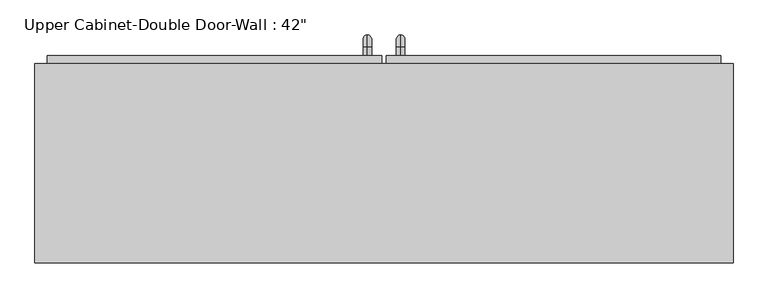
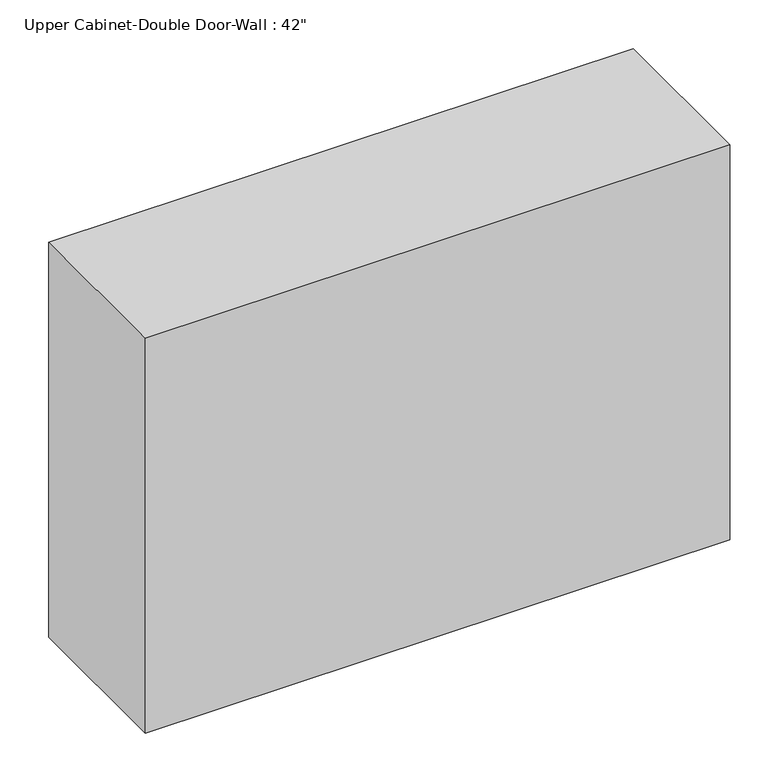
"""IFC4 building model written with IfcOpenShell, lengths in millimetres: furniture geometry."""

from ifc_helpers import new_model, si_unit, point, frame, origin, place, context, project, spatial, polyline, circle_curve, ellipse_curve, trimmed, outline, extrude, faceted_brep, source, transform, mapped, element, save
from ifc_brep_helpers import plane_surface, cylinder_surface, revolved_surface, advanced_brep


def furniture_f73e1c42(model_context):
    return source(origin(), model_context, "Body", "SolidModel", [
        extrude(outline(polyline([(32.9461628, 374.65), (544.1211628, 374.65), (544.1211628, 342.9), (32.9461628, 342.9), (32.9461628, 374.65)])), frame((0.0, 0.0, 1390.65), z_axis=(0.0, 0.0, 1.0), x_axis=(1.0, 0.0, 0.0)), (0.0, 0.0, 1.0), 723.9),
        extrude(outline(polyline([(-484.5788372, 374.65), (26.5961628, 374.65), (26.5961628, 342.9), (-484.5788372, 342.9), (-484.5788372, 374.65)])), frame((0.0, 0.0, 1390.65), z_axis=(0.0, 0.0, 1.0), x_axis=(1.0, 0.0, 0.0)), (0.0, 0.0, 1.0), 723.9),
        advanced_brep(
        [(4.3711628, 374.65, 1517.65), (4.3711628, 374.65, 1530.35), (4.3711628, 387.35, 1517.65), (4.3711628, 387.35, 1530.35), (4.3711628, 406.4, 1511.3), (4.3711628, 393.7, 1511.3), (4.3711628, 393.7, 1435.1), (4.3711628, 406.4, 1435.1), (4.3711628, 387.35, 1416.05), (4.3711628, 387.35, 1428.75), (4.3711628, 374.65, 1428.75), (4.3711628, 374.65, 1416.05)],
        [
            (0, 1, circle_curve(frame((4.3711628, 374.65, 1524.0), z_axis=(0.0, -1.0, 0.0), x_axis=(0.0, 0.0, 1.0)), 6.35)),
            (1, 0, circle_curve(frame((4.3711628, 374.65, 1524.0), z_axis=(0.0, -1.0, 0.0), x_axis=(0.0, 0.0, 1.0)), 6.35)),
            (0, 2),
            (2, 3, circle_curve(frame((4.3711628, 387.35, 1524.0), z_axis=(0.0, -1.0, 0.0), x_axis=(0.0, 0.0, 1.0)), 6.35)),
            (3, 1),
            (3, 2, circle_curve(frame((4.3711628, 387.35, 1524.0), z_axis=(0.0, -1.0, 0.0), x_axis=(0.0, 0.0, 1.0)), 6.35)),
            (4, 3, circle_curve(frame((4.3711628, 387.35, 1511.3), z_axis=(1.0, 0.0, 0.0), x_axis=(0.0, 0.0, 1.0)), 19.05)),
            (2, 5, circle_curve(frame((4.3711628, 387.35, 1511.3), z_axis=(-1.0, 0.0, 0.0), x_axis=(0.0, 0.0, 1.0)), 6.35)),
            (5, 4, circle_curve(frame((4.3711628, 400.05, 1511.3), z_axis=(0.0, 0.0, 1.0), x_axis=(0.0, 1.0, 0.0)), 6.35)),
            (4, 5, circle_curve(frame((4.3711628, 400.05, 1511.3), z_axis=(0.0, 0.0, 1.0), x_axis=(0.0, 1.0, 0.0)), 6.35)),
            (5, 6),
            (6, 7, circle_curve(frame((4.3711628, 400.05, 1435.1), z_axis=(0.0, 0.0, 1.0), x_axis=(0.0, 1.0, 0.0)), 6.35)),
            (7, 4),
            (7, 6, circle_curve(frame((4.3711628, 400.05, 1435.1), z_axis=(0.0, 0.0, 1.0), x_axis=(0.0, 1.0, 0.0)), 6.35)),
            (8, 7, circle_curve(frame((4.3711628, 387.35, 1435.1), z_axis=(1.0, 0.0, 0.0), x_axis=(0.0, 1.0, 0.0)), 19.05)),
            (6, 9, circle_curve(frame((4.3711628, 387.35, 1435.1), z_axis=(-1.0, 0.0, 0.0), x_axis=(0.0, 1.0, 0.0)), 6.35)),
            (9, 8, circle_curve(frame((4.3711628, 387.35, 1422.4), z_axis=(0.0, 1.0, 0.0), x_axis=(0.0, 0.0, -1.0)), 6.35)),
            (8, 9, circle_curve(frame((4.3711628, 387.35, 1422.4), z_axis=(0.0, 1.0, 0.0), x_axis=(0.0, 0.0, -1.0)), 6.35)),
            (10, 11, circle_curve(frame((4.3711628, 374.65, 1422.4), z_axis=(0.0, -1.0, 0.0), x_axis=(0.0, 0.0, -1.0)), 6.35)),
            (11, 10, circle_curve(frame((4.3711628, 374.65, 1422.4), z_axis=(0.0, -1.0, 0.0), x_axis=(0.0, 0.0, -1.0)), 6.35)),
            (9, 10),
            (11, 8),
        ],
        [
            plane_surface(frame((-1.9788372, 374.65, 1524.0), z_axis=(0.0, -1.0, 0.0), x_axis=(0.0, 0.0, 1.0))),
            cylinder_surface(frame((4.3711628, 374.65, 1524.0), z_axis=(0.0, -1.0, 0.0), x_axis=(0.0, 0.0, 1.0)), 6.35),
            revolved_surface(trimmed(ellipse_curve(frame((4.3711628, 387.35, 1524.0), z_axis=(0.0, -1.0, 0.0), x_axis=(0.0, 0.0, 1.0)), 6.35, 6.35), [point((4.3711628, 387.35, 1517.65))], [point((4.3711628, 387.35, 1530.35))], True, "CARTESIAN"), (4.3711628, 387.35, 1511.3), (-1.0, 0.0, 0.0)),
            revolved_surface(trimmed(ellipse_curve(frame((4.3711628, 387.35, 1524.0), z_axis=(0.0, -1.0, 0.0), x_axis=(0.0, 0.0, 1.0)), 6.35, 6.35), [point((4.3711628, 387.35, 1530.35))], [point((4.3711628, 387.35, 1517.65))], True, "CARTESIAN"), (4.3711628, 387.35, 1511.3), (-1.0, 0.0, 0.0)),
            cylinder_surface(frame((4.3711628, 400.05, 1511.3), z_axis=(0.0, 0.0, 1.0), x_axis=(0.0, 1.0, 0.0)), 6.35),
            revolved_surface(trimmed(ellipse_curve(frame((4.3711628, 400.05, 1435.1), z_axis=(0.0, 0.0, 1.0), x_axis=(0.0, 1.0, 0.0)), 6.35, 6.35), [point((4.3711628, 393.7, 1435.1))], [point((4.3711628, 406.4, 1435.1))], True, "CARTESIAN"), (4.3711628, 387.35, 1435.1), (-1.0, 0.0, 0.0)),
            revolved_surface(trimmed(ellipse_curve(frame((4.3711628, 400.05, 1435.1), z_axis=(0.0, 0.0, 1.0), x_axis=(0.0, 1.0, 0.0)), 6.35, 6.35), [point((4.3711628, 406.4, 1435.1))], [point((4.3711628, 393.7, 1435.1))], True, "CARTESIAN"), (4.3711628, 387.35, 1435.1), (-1.0, 0.0, 0.0)),
            plane_surface(frame((-1.9788372, 374.65, 1422.4), z_axis=(0.0, -1.0, 0.0), x_axis=(0.0, 0.0, -1.0))),
            cylinder_surface(frame((4.3711628, 387.35, 1422.4), z_axis=(0.0, 1.0, 0.0), x_axis=(0.0, 0.0, -1.0)), 6.35),
        ],
        [
            (0, [[1, 2]]),
            (1, [[-1, 3, 4, 5]]),
            (1, [[-2, -5, 6, -3]]),
            (2, [[7, -4, 8, 9]]),
            (3, [[-8, -6, -7, 10]]),
            (4, [[-9, 11, 12, 13]]),
            (4, [[-10, -13, 14, -11]]),
            (5, [[15, -12, 16, 17]]),
            (6, [[-16, -14, -15, 18]]),
            (7, [[19, 20]]),
            (8, [[-17, 21, -20, 22]]),
            (8, [[-18, -22, -19, -21]]),
        ],
    ),
        advanced_brep(
        [(55.1711628, 374.65, 1517.65), (55.1711628, 374.65, 1530.35), (55.1711628, 387.35, 1517.65), (55.1711628, 387.35, 1530.35), (55.1711628, 406.4, 1511.3), (55.1711628, 393.7, 1511.3), (55.1711628, 393.7, 1435.1), (55.1711628, 406.4, 1435.1), (55.1711628, 387.35, 1416.05), (55.1711628, 387.35, 1428.75), (55.1711628, 374.65, 1428.75), (55.1711628, 374.65, 1416.05)],
        [
            (0, 1, circle_curve(frame((55.1711628, 374.65, 1524.0), z_axis=(0.0, -1.0, 0.0), x_axis=(0.0, 0.0, -1.0)), 6.35)),
            (1, 0, circle_curve(frame((55.1711628, 374.65, 1524.0), z_axis=(0.0, -1.0, 0.0), x_axis=(0.0, 0.0, -1.0)), 6.35)),
            (0, 2),
            (2, 3, circle_curve(frame((55.1711628, 387.35, 1524.0), z_axis=(0.0, -1.0, 0.0), x_axis=(0.0, 0.0, -1.0)), 6.35)),
            (3, 1),
            (3, 2, circle_curve(frame((55.1711628, 387.35, 1524.0), z_axis=(0.0, -1.0, 0.0), x_axis=(0.0, 0.0, -1.0)), 6.35)),
            (4, 3, circle_curve(frame((55.1711628, 387.35, 1511.3), z_axis=(1.0, 0.0, 0.0), x_axis=(0.0, 0.0, 1.0)), 19.05)),
            (2, 5, circle_curve(frame((55.1711628, 387.35, 1511.3), z_axis=(-1.0, 0.0, 0.0), x_axis=(0.0, 0.0, 1.0)), 6.35)),
            (5, 4, circle_curve(frame((55.1711628, 400.05, 1511.3), z_axis=(0.0, 0.0, 1.0), x_axis=(0.0, -1.0, 0.0)), 6.35)),
            (4, 5, circle_curve(frame((55.1711628, 400.05, 1511.3), z_axis=(0.0, 0.0, 1.0), x_axis=(0.0, -1.0, 0.0)), 6.35)),
            (5, 6),
            (6, 7, circle_curve(frame((55.1711628, 400.05, 1435.1), z_axis=(0.0, 0.0, 1.0), x_axis=(0.0, -1.0, 0.0)), 6.35)),
            (7, 4),
            (7, 6, circle_curve(frame((55.1711628, 400.05, 1435.1), z_axis=(0.0, 0.0, 1.0), x_axis=(0.0, -1.0, 0.0)), 6.35)),
            (8, 7, circle_curve(frame((55.1711628, 387.35, 1435.1), z_axis=(1.0, 0.0, 0.0), x_axis=(0.0, 1.0, 0.0)), 19.05)),
            (6, 9, circle_curve(frame((55.1711628, 387.35, 1435.1), z_axis=(-1.0, 0.0, 0.0), x_axis=(0.0, 1.0, 0.0)), 6.35)),
            (9, 8, circle_curve(frame((55.1711628, 387.35, 1422.4), z_axis=(0.0, 1.0, 0.0), x_axis=(0.0, 0.0, 1.0)), 6.35)),
            (8, 9, circle_curve(frame((55.1711628, 387.35, 1422.4), z_axis=(0.0, 1.0, 0.0), x_axis=(0.0, 0.0, 1.0)), 6.35)),
            (10, 11, circle_curve(frame((55.1711628, 374.65, 1422.4), z_axis=(0.0, -1.0, 0.0), x_axis=(0.0, 0.0, 1.0)), 6.35)),
            (11, 10, circle_curve(frame((55.1711628, 374.65, 1422.4), z_axis=(0.0, -1.0, 0.0), x_axis=(0.0, 0.0, 1.0)), 6.35)),
            (9, 10),
            (11, 8),
        ],
        [
            plane_surface(frame((48.8211628, 374.65, 1524.0), z_axis=(0.0, -1.0, 0.0), x_axis=(0.0, 0.0, 1.0))),
            cylinder_surface(frame((55.1711628, 374.65, 1524.0), z_axis=(0.0, -1.0, 0.0), x_axis=(0.0, 0.0, -1.0)), 6.35),
            revolved_surface(trimmed(ellipse_curve(frame((55.1711628, 387.35, 1524.0), z_axis=(0.0, -1.0, 0.0), x_axis=(0.0, 0.0, -1.0)), 6.35, 6.35), [point((55.1711628, 387.35, 1517.65))], [point((55.1711628, 387.35, 1530.35))], True, "CARTESIAN"), (55.1711628, 387.35, 1511.3), (-1.0, 0.0, 0.0)),
            revolved_surface(trimmed(ellipse_curve(frame((55.1711628, 387.35, 1524.0), z_axis=(0.0, -1.0, 0.0), x_axis=(0.0, 0.0, -1.0)), 6.35, 6.35), [point((55.1711628, 387.35, 1530.35))], [point((55.1711628, 387.35, 1517.65))], True, "CARTESIAN"), (55.1711628, 387.35, 1511.3), (-1.0, 0.0, 0.0)),
            cylinder_surface(frame((55.1711628, 400.05, 1511.3), z_axis=(0.0, 0.0, 1.0), x_axis=(0.0, -1.0, 0.0)), 6.35),
            revolved_surface(trimmed(ellipse_curve(frame((55.1711628, 400.05, 1435.1), z_axis=(0.0, 0.0, 1.0), x_axis=(0.0, -1.0, 0.0)), 6.35, 6.35), [point((55.1711628, 393.7, 1435.1))], [point((55.1711628, 406.4, 1435.1))], True, "CARTESIAN"), (55.1711628, 387.35, 1435.1), (-1.0, 0.0, 0.0)),
            revolved_surface(trimmed(ellipse_curve(frame((55.1711628, 400.05, 1435.1), z_axis=(0.0, 0.0, 1.0), x_axis=(0.0, -1.0, 0.0)), 6.35, 6.35), [point((55.1711628, 406.4, 1435.1))], [point((55.1711628, 393.7, 1435.1))], True, "CARTESIAN"), (55.1711628, 387.35, 1435.1), (-1.0, 0.0, 0.0)),
            plane_surface(frame((48.8211628, 374.65, 1422.4), z_axis=(0.0, -1.0, 0.0), x_axis=(0.0, 0.0, -1.0))),
            cylinder_surface(frame((55.1711628, 387.35, 1422.4), z_axis=(0.0, 1.0, 0.0), x_axis=(0.0, 0.0, 1.0)), 6.35),
        ],
        [
            (0, [[1, 2]]),
            (1, [[-1, 3, 4, 5]]),
            (1, [[-2, -5, 6, -3]]),
            (2, [[7, -4, 8, 9]]),
            (3, [[-8, -6, -7, 10]]),
            (4, [[-9, 11, 12, 13]]),
            (4, [[-10, -13, 14, -11]]),
            (5, [[15, -12, 16, 17]]),
            (6, [[-16, -14, -15, 18]]),
            (7, [[19, 20]]),
            (8, [[-17, 21, -20, 22]]),
            (8, [[-18, -22, -19, -21]]),
        ],
    ),
        faceted_brep([(-503.6288372, 57.15, 2133.6), (-503.6288372, 57.15, 1371.6), (563.1711628, 57.15, 1371.6), (563.1711628, 57.15, 2133.6), (-503.6288372, 361.95, 2133.6), (563.1711628, 361.95, 2133.6), (563.1711628, 361.95, 1371.6), (-503.6288372, 361.95, 1371.6), (-484.5788372, 361.95, 2114.55), (-484.5788372, 361.95, 1390.65), (544.1211628, 361.95, 1390.65), (544.1211628, 361.95, 2114.55), (544.1211628, 76.2, 2114.55), (-484.5788372, 76.2, 2114.55), (544.1211628, 76.2, 1390.65), (-484.5788372, 76.2, 1390.65)], [[[0, 1, 2, 3]], [[4, 5, 6, 7], [8, 9, 10, 11]], [[1, 0, 4, 7]], [[2, 1, 7, 6]], [[3, 2, 6, 5]], [[0, 3, 5, 4]], [[8, 11, 12, 13]], [[11, 10, 14, 12]], [[10, 9, 15, 14]], [[9, 8, 13, 15]], [[13, 12, 14, 15]]]),
    ])


if __name__ == "__main__":
    model = new_model("IFC4")
    model_context = context("Model", 3, world=origin())
    ifc_project = project(units=[si_unit("LENGTHUNIT", "METRE", prefix="MILLI")], contexts=[model_context])
    site = spatial("IfcSite", under=ifc_project)
    building = spatial("IfcBuilding", under=site)
    placement = place(None, origin())
    furniture_shape = furniture_f73e1c42(model_context)
    element("IfcFurniture", 1, ObjectType="Upper Cabinet-Double Door-Wall : 42\"", at=placement, inside=building, context=model_context, shape_type="MappedRepresentation", body=[
        mapped(furniture_shape, transform((0.0, 0.0, 0.0), x_axis=(1.0, 0.0, 0.0), y_axis=(0.0, 1.0, 0.0), z_axis=(0.0, 0.0, 1.0))),
    ])
    save(model, "model.ifc")

# Revit data of these elements
# Type "Upper Cabinet-Double Door-Wall : 42\""
#   Assembly Code = "C1030410"
#   Depth = 1' - 0"
#   Height = 2' - 6"
#   Top Of Cabinet = 7' - 0"
#   Width = 3' - 6"
#   Cabinet Material = none
#   Door/Drawer Material = none
#   Handle Material = Cabinets - Handles
#   Default Elevation = 0
# Element 1 (IfcFurniture, "Upper Cabinet-Double Door-Wall : 42\"")
#   Materials on its faces: "Cabinets - Handles", "Cabinet"
# Materials
#   "Cabinets - Handles": colour RGB 57 57 57, transparency 0
#   "Cabinet": colour RGB 204 122 2, transparency 0
